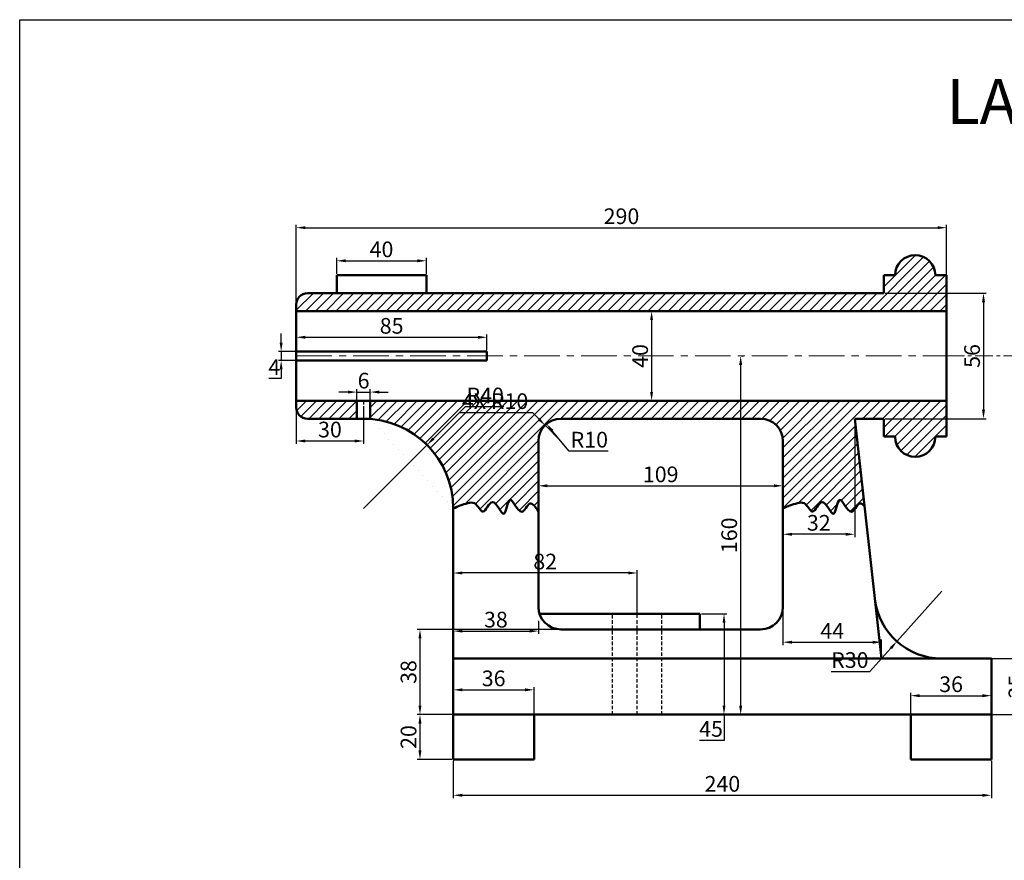
# Model space of a CAD drawing. Units: millimetres. Extents: x -66 to 1195, y -396 to 398.
# Tile 2 of 8: x -66 to 373, y 23 to 398. Entities that reach past the tile are written whole.
import ezdxf

# ---------------------------------------------------------------- set-up
doc = ezdxf.new("R2010")
doc.units = ezdxf.units.MM
doc.header["$LTSCALE"] = 0.5
doc.linetypes.add('CENTER', pattern=[50.8, 31.75, -6.35, 6.35, -6.35])
doc.linetypes.add('HIDDEN', pattern=[9.525, 6.35, -3.175])
for name, color, linetype, lineweight in [('M-CNTR', 1, 'CENTER', 18), ('M-DIMS', 2, 'Continuous', 25), ('M-HATC', 8, 'Continuous', 18), ('M-HIDN', 3, 'HIDDEN', 25), ('M-OUTL', 7, 'Continuous', 50), ('M-TEXT', 7, 'Continuous', 25), ('M-TTLB', 7, 'Continuous', 25)]:
    doc.layers.add(name, color=color, linetype=linetype, lineweight=lineweight)
doc.styles.get("Standard").update_dxf_attribs({"font": 'arial.ttf'})
doc.dimstyles.new('ISO-25', dxfattribs={"dimtxt": 7, "dimasz": 4, "dimexe": 1.25, "dimexo": 0.625, "dimtad": 1, "dimtoh": 1, "dimtxsty": 'Standard', "dimcen": 2.5, "dimadec": 0, "dimazin": 0, "dimtfac": 1, "dimtmove": 0, "dimatfit": 3, "dimfxl": 1, "dimarcsym": 0})

# ---------------------------------------------------------------- blocks, each defined once
blk = doc.blocks.new('*D1')
at = {"layer": 'Defpoints', "color": 0, "ltscale": 0.5, "transparency": 16777216}
for p in [(114.94, 290.08), (74.94, 283.61), (114.94, 283.61)]:
    blk.add_point(p, dxfattribs=at)
at = {"layer": 'M-DIMS', "color": 0, "lineweight": -2, "ltscale": 0.5, "transparency": 16777216}
for p, q in [((74.94, 284.24), (74.94, 291.33)), ((78.94, 290.08), (110.94, 290.08)), ((114.94, 284.24), (114.94, 291.33))]:
    blk.add_line(p, q, dxfattribs=at)
at = {"layer": 'M-DIMS', "color": 0, "ltscale": 0.5, "transparency": 16777216}
for points in [[(78.94, 290.75), (78.94, 289.41), (74.94, 290.08)], [(110.94, 290.75), (110.94, 289.41), (114.94, 290.08)]]:
    blk.add_solid(points, dxfattribs=at)
at = {"layer": 'M-DIMS', "color": 0, "ltscale": 0.5, "transparency": 16777216, "insert": (94.94, 294.28), "char_height": 7, "attachment_point": 5}
blk.add_mtext('40', dxfattribs=at)
blk = doc.blocks.new('*D2')
at = {"layer": 'Defpoints', "color": 0, "ltscale": 0.5, "transparency": 16777216}
for p in [(346.94, 304.84), (56.94, 249.61), (346.94, 247.61)]:
    blk.add_point(p, dxfattribs=at)
at = {"layer": 'M-DIMS', "color": 0, "lineweight": -2, "ltscale": 0.5, "transparency": 16777216}
for p, q in [((56.94, 250.24), (56.94, 306.09)), ((60.94, 304.84), (342.94, 304.84)), ((346.94, 248.24), (346.94, 306.09))]:
    blk.add_line(p, q, dxfattribs=at)
at = {"layer": 'M-DIMS', "color": 0, "ltscale": 0.5, "transparency": 16777216}
for points in [[(60.94, 305.51), (60.94, 304.18), (56.94, 304.84)], [(342.94, 305.51), (342.94, 304.18), (346.94, 304.84)]]:
    blk.add_solid(points, dxfattribs=at)
at = {"layer": 'M-DIMS', "color": 0, "ltscale": 0.5, "transparency": 16777216, "insert": (201.94, 309.04), "char_height": 7, "attachment_point": 5}
blk.add_mtext('290', dxfattribs=at)
blk = doc.blocks.new('*D3')
at = {"layer": 'Defpoints', "color": 0, "ltscale": 0.5, "transparency": 16777216}
for p in [(141.94, 255.95), (56.94, 249.61), (141.94, 249.61)]:
    blk.add_point(p, dxfattribs=at)
at = {"layer": 'M-DIMS', "color": 0, "lineweight": -2, "ltscale": 0.5, "transparency": 16777216}
for p, q in [((56.94, 250.24), (56.94, 257.2)), ((60.94, 255.95), (137.94, 255.95)), ((141.94, 250.24), (141.94, 257.2))]:
    blk.add_line(p, q, dxfattribs=at)
at = {"layer": 'M-DIMS', "color": 0, "ltscale": 0.5, "transparency": 16777216}
for points in [[(60.94, 256.61), (60.94, 255.28), (56.94, 255.95)], [(137.94, 256.61), (137.94, 255.28), (141.94, 255.95)]]:
    blk.add_solid(points, dxfattribs=at)
at = {"layer": 'M-DIMS', "color": 0, "ltscale": 0.5, "transparency": 16777216, "insert": (99.44, 260.15), "char_height": 7, "attachment_point": 5}
blk.add_mtext('85', dxfattribs=at)
blk = doc.blocks.new('*D4')
at = {"layer": 'Defpoints', "color": 0, "ltscale": 0.5, "transparency": 16777216}
for p in [(56.94, 249.61), (50.18, 245.61), (56.94, 245.61)]:
    blk.add_point(p, dxfattribs=at)
at = {"layer": 'M-DIMS', "color": 0, "lineweight": -2, "ltscale": 0.5, "transparency": 16777216}
for p, q in [((50.18, 253.61), (50.18, 257.61)), ((56.31, 249.61), (48.93, 249.61)), ((50.18, 249.61), (50.18, 245.61)), ((56.31, 245.61), (48.93, 245.61)), ((50.18, 241.61), (50.18, 237.61)), ((50.18, 237.61), (44.71, 237.61))]:
    blk.add_line(p, q, dxfattribs=at)
at = {"layer": 'M-DIMS', "color": 0, "ltscale": 0.5, "transparency": 16777216}
for points in [[(49.51, 253.61), (50.84, 253.61), (50.18, 249.61)], [(49.51, 241.61), (50.84, 241.61), (50.18, 245.61)]]:
    blk.add_solid(points, dxfattribs=at)
at = {"layer": 'M-DIMS', "color": 0, "ltscale": 0.5, "transparency": 16777216, "insert": (47.13, 241.74), "char_height": 7, "attachment_point": 5}
blk.add_mtext('4', dxfattribs=at)
blk = doc.blocks.new('*D5')
at = {"layer": 'Defpoints', "color": 0, "ltscale": 0.5, "transparency": 16777216}
for p in [(219.72, 267.61), (215.38, 227.61), (219.72, 227.61)]:
    blk.add_point(p, dxfattribs=at)
at = {"layer": 'M-DIMS', "color": 0, "lineweight": -2, "ltscale": 0.5, "transparency": 16777216}
for p, q in [((219.09, 267.61), (214.13, 267.61)), ((215.38, 263.61), (215.38, 231.61)), ((219.09, 227.61), (214.13, 227.61))]:
    blk.add_line(p, q, dxfattribs=at)
at = {"layer": 'M-DIMS', "color": 0, "ltscale": 0.5, "transparency": 16777216}
for points in [[(214.71, 263.61), (216.04, 263.61), (215.38, 267.61)], [(214.71, 231.61), (216.04, 231.61), (215.38, 227.61)]]:
    blk.add_solid(points, dxfattribs=at)
at = {"layer": 'M-DIMS', "color": 0, "ltscale": 0.5, "transparency": 16777216, "insert": (211.18, 247.61), "char_height": 7, "attachment_point": 5, "rotation": 90}
blk.add_mtext('40', dxfattribs=at)
blk = doc.blocks.new('*D6')
at = {"layer": 'Defpoints', "color": 0, "ltscale": 0.5, "transparency": 16777216}
for p in [(56.94, 224.61), (86.94, 224.61), (86.94, 209.68)]:
    blk.add_point(p, dxfattribs=at)
at = {"layer": 'M-DIMS', "color": 0, "lineweight": -2, "ltscale": 0.5, "transparency": 16777216}
for p, q in [((56.94, 223.99), (56.94, 208.43)), ((86.94, 223.99), (86.94, 208.43)), ((60.94, 209.68), (82.94, 209.68))]:
    blk.add_line(p, q, dxfattribs=at)
at = {"layer": 'M-DIMS', "color": 0, "ltscale": 0.5, "transparency": 16777216}
for points in [[(60.94, 210.35), (60.94, 209.01), (56.94, 209.68)], [(82.94, 210.35), (82.94, 209.01), (86.94, 209.68)]]:
    blk.add_solid(points, dxfattribs=at)
at = {"layer": 'M-DIMS', "color": 0, "ltscale": 0.5, "transparency": 16777216, "insert": (71.94, 213.88), "char_height": 7, "attachment_point": 5}
blk.add_mtext('30', dxfattribs=at)
blk = doc.blocks.new('*D7')
at = {"layer": 'Defpoints', "color": 0, "ltscale": 0.5, "transparency": 16777216}
for p in [(89.94, 231.5), (83.94, 227.61), (89.94, 227.61)]:
    blk.add_point(p, dxfattribs=at)
at = {"layer": 'M-DIMS', "color": 0, "lineweight": -2, "ltscale": 0.5, "transparency": 16777216}
for p, q in [((83.94, 228.24), (83.94, 232.75)), ((89.94, 228.24), (89.94, 232.75)), ((79.94, 231.5), (75.94, 231.5)), ((83.94, 231.5), (89.94, 231.5)), ((93.94, 231.5), (97.94, 231.5))]:
    blk.add_line(p, q, dxfattribs=at)
at = {"layer": 'M-DIMS', "color": 0, "ltscale": 0.5, "transparency": 16777216}
for points in [[(79.94, 232.17), (79.94, 230.84), (83.94, 231.5)], [(93.94, 232.17), (93.94, 230.84), (89.94, 231.5)]]:
    blk.add_solid(points, dxfattribs=at)
at = {"layer": 'M-DIMS', "color": 0, "ltscale": 0.5, "transparency": 16777216, "insert": (86.94, 235.7), "char_height": 7, "attachment_point": 5}
blk.add_mtext('6', dxfattribs=at)
blk = doc.blocks.new('*D8')
at = {"layer": 'Defpoints', "color": 0, "ltscale": 0.5, "transparency": 16777216}
for p in [(305.94, 219.61), (273.94, 199.66), (273.94, 168.06)]:
    blk.add_point(p, dxfattribs=at)
at = {"layer": 'M-DIMS', "color": 0, "lineweight": -2, "ltscale": 0.5, "transparency": 16777216}
for p, q in [((305.94, 218.99), (305.94, 166.81)), ((273.94, 199.04), (273.94, 166.81)), ((301.94, 168.06), (277.94, 168.06))]:
    blk.add_line(p, q, dxfattribs=at)
at = {"layer": 'M-DIMS', "color": 0, "ltscale": 0.5, "transparency": 16777216}
for points in [[(277.94, 168.73), (277.94, 167.39), (273.94, 168.06)], [(301.94, 168.73), (301.94, 167.39), (305.94, 168.06)]]:
    blk.add_solid(points, dxfattribs=at)
at = {"layer": 'M-DIMS', "color": 0, "ltscale": 0.5, "transparency": 16777216, "insert": (289.94, 172.26), "char_height": 7, "attachment_point": 5}
blk.add_mtext('32', dxfattribs=at)
blk = doc.blocks.new('*D9')
at = {"layer": 'Defpoints', "color": 0, "ltscale": 0.5, "transparency": 16777216}
for p in [(273.94, 142.91), (317.94, 119.9), (317.94, 112.61)]:
    blk.add_point(p, dxfattribs=at)
at = {"layer": 'M-DIMS', "color": 0, "lineweight": -2, "ltscale": 0.5, "transparency": 16777216}
for p, q in [((273.94, 142.29), (273.94, 118.65)), ((277.94, 119.9), (313.94, 119.9)), ((317.94, 113.24), (317.94, 121.15))]:
    blk.add_line(p, q, dxfattribs=at)
at = {"layer": 'M-DIMS', "color": 0, "ltscale": 0.5, "transparency": 16777216}
for points in [[(277.94, 120.57), (277.94, 119.24), (273.94, 119.9)], [(313.94, 120.57), (313.94, 119.24), (317.94, 119.9)]]:
    blk.add_solid(points, dxfattribs=at)
at = {"layer": 'M-DIMS', "color": 0, "ltscale": 0.5, "transparency": 16777216, "insert": (295.94, 124.03), "char_height": 7, "attachment_point": 5}
blk.add_mtext('44', dxfattribs=at)
blk = doc.blocks.new('*D10')
at = {"layer": 'Defpoints', "color": 0, "ltscale": 0.5, "transparency": 16777216}
for p in [(126.94, 150.79), (126.94, 130.11), (208.94, 130.11)]:
    blk.add_point(p, dxfattribs=at)
at = {"layer": 'M-DIMS', "color": 0, "lineweight": -2, "ltscale": 0.5, "transparency": 16777216}
for p, q in [((126.94, 130.74), (126.94, 152.04)), ((204.94, 150.79), (130.94, 150.79)), ((208.94, 130.74), (208.94, 152.04))]:
    blk.add_line(p, q, dxfattribs=at)
at = {"layer": 'M-DIMS', "color": 0, "ltscale": 0.5, "transparency": 16777216}
for points in [[(130.94, 151.46), (130.94, 150.12), (126.94, 150.79)], [(204.94, 151.46), (204.94, 150.12), (208.94, 150.79)]]:
    blk.add_solid(points, dxfattribs=at)
at = {"layer": 'M-DIMS', "color": 0, "ltscale": 0.5, "transparency": 16777216, "insert": (167.94, 154.99), "char_height": 7, "attachment_point": 5}
blk.add_mtext('82', dxfattribs=at)
blk = doc.blocks.new('*D11')
at = {"layer": 'Defpoints', "color": 0, "ltscale": 0.5, "transparency": 16777216}
for p in [(126.94, 130.11), (164.94, 130.11), (164.94, 124.87)]:
    blk.add_point(p, dxfattribs=at)
at = {"layer": 'M-DIMS', "color": 0, "lineweight": -2, "ltscale": 0.5, "transparency": 16777216}
for p, q in [((126.94, 129.49), (126.94, 123.62)), ((164.94, 129.49), (164.94, 123.62)), ((130.94, 124.87), (160.94, 124.87))]:
    blk.add_line(p, q, dxfattribs=at)
at = {"layer": 'M-DIMS', "color": 0, "ltscale": 0.5, "transparency": 16777216}
for points in [[(130.94, 125.53), (130.94, 124.2), (126.94, 124.87)], [(160.94, 125.53), (160.94, 124.2), (164.94, 124.87)]]:
    blk.add_solid(points, dxfattribs=at)
at = {"layer": 'M-DIMS', "color": 0, "ltscale": 0.5, "transparency": 16777216, "insert": (145.94, 129.07), "char_height": 7, "attachment_point": 5}
blk.add_mtext('38', dxfattribs=at)
blk = doc.blocks.new('*D12')
at = {"layer": 'Defpoints', "color": 0, "ltscale": 0.5, "transparency": 16777216}
for p in [(254.81, 247.61), (254.81, 87.61), (255.09, 87.61)]:
    blk.add_point(p, dxfattribs=at)
at = {"layer": 'M-DIMS', "color": 0, "lineweight": -2, "ltscale": 0.5, "transparency": 16777216}
for p, q in [((255.43, 247.61), (256.34, 247.61)), ((255.09, 243.61), (255.09, 91.61)), ((255.43, 87.61), (256.34, 87.61))]:
    blk.add_line(p, q, dxfattribs=at)
at = {"layer": 'M-DIMS', "color": 0, "ltscale": 0.5, "transparency": 16777216}
for points in [[(254.42, 243.61), (255.76, 243.61), (255.09, 247.61)], [(254.42, 91.61), (255.76, 91.61), (255.09, 87.61)]]:
    blk.add_solid(points, dxfattribs=at)
at = {"layer": 'M-DIMS', "color": 0, "ltscale": 0.5, "transparency": 16777216, "insert": (250.89, 167.61), "char_height": 7, "attachment_point": 5, "rotation": 90}
blk.add_mtext('160', dxfattribs=at)
blk = doc.blocks.new('*D13')
at = {"layer": 'Defpoints', "color": 0, "ltscale": 0.5, "transparency": 16777216}
for p in [(273.94, 189.69), (164.94, 188.31), (273.94, 188.31)]:
    blk.add_point(p, dxfattribs=at)
at = {"layer": 'M-DIMS', "color": 0, "lineweight": -2, "ltscale": 0.5, "transparency": 16777216}
for p, q in [((164.94, 188.93), (164.94, 190.94)), ((168.94, 189.69), (269.94, 189.69)), ((273.94, 188.93), (273.94, 190.94))]:
    blk.add_line(p, q, dxfattribs=at)
at = {"layer": 'M-DIMS', "color": 0, "ltscale": 0.5, "transparency": 16777216}
for points in [[(168.94, 190.35), (168.94, 189.02), (164.94, 189.69)], [(269.94, 190.35), (269.94, 189.02), (273.94, 189.69)]]:
    blk.add_solid(points, dxfattribs=at)
at = {"layer": 'M-DIMS', "color": 0, "ltscale": 0.5, "transparency": 16777216, "insert": (219.44, 193.89), "char_height": 7, "attachment_point": 5}
blk.add_mtext('109', dxfattribs=at)
blk = doc.blocks.new('*D14')
at = {"layer": 'Defpoints', "color": 0, "ltscale": 0.5, "transparency": 16777216}
for p in [(168.54, 217.3), (174.94, 209.61)]:
    blk.add_point(p, dxfattribs=at)
at = {"layer": 'M-DIMS', "color": 0, "lineweight": -2, "ltscale": 0.5, "transparency": 16777216}
for p, q in [((178.64, 205.16), (171.1, 214.22)), ((195.96, 205.16), (178.64, 205.16))]:
    blk.add_line(p, q, dxfattribs=at)
at = {"layer": 'M-DIMS', "color": 0, "ltscale": 0.5, "transparency": 16777216}
blk.add_solid([(171.61, 214.65), (170.59, 213.8), (168.54, 217.3)], dxfattribs=at)
at = {"layer": 'M-DIMS', "color": 0, "ltscale": 0.5, "transparency": 16777216, "insert": (187.61, 209.36), "char_height": 7, "attachment_point": 5}
blk.add_mtext('R10', dxfattribs=at)
blk = doc.blocks.new('*D15')
at = {"layer": 'Defpoints', "color": 0, "ltscale": 0.5, "transparency": 16777216}
for p in [(181.38, 125.61), (112.09, 87.61), (181.38, 87.61)]:
    blk.add_point(p, dxfattribs=at)
at = {"layer": 'M-DIMS', "color": 0, "lineweight": -2, "ltscale": 0.5, "transparency": 16777216}
for p, q in [((180.75, 125.61), (110.84, 125.61)), ((112.09, 121.61), (112.09, 91.61)), ((180.75, 87.61), (110.84, 87.61))]:
    blk.add_line(p, q, dxfattribs=at)
at = {"layer": 'M-DIMS', "color": 0, "ltscale": 0.5, "transparency": 16777216}
for points in [[(111.42, 121.61), (112.75, 121.61), (112.09, 125.61)], [(111.42, 91.61), (112.75, 91.61), (112.09, 87.61)]]:
    blk.add_solid(points, dxfattribs=at)
at = {"layer": 'M-DIMS', "color": 0, "ltscale": 0.5, "transparency": 16777216, "insert": (107.89, 106.61), "char_height": 7, "attachment_point": 5, "rotation": 90}
blk.add_mtext('38', dxfattribs=at)
blk = doc.blocks.new('*D16')
at = {"layer": 'Defpoints', "color": 0, "ltscale": 0.5, "transparency": 16777216}
for p in [(126.94, 87.61), (112.09, 67.61), (126.94, 67.61)]:
    blk.add_point(p, dxfattribs=at)
at = {"layer": 'M-DIMS', "color": 0, "lineweight": -2, "ltscale": 0.5, "transparency": 16777216}
for p, q in [((126.31, 87.61), (110.84, 87.61)), ((112.09, 83.61), (112.09, 71.61)), ((126.31, 67.61), (110.84, 67.61))]:
    blk.add_line(p, q, dxfattribs=at)
at = {"layer": 'M-DIMS', "color": 0, "ltscale": 0.5, "transparency": 16777216}
for points in [[(111.42, 83.61), (112.75, 83.61), (112.09, 87.61)], [(111.42, 71.61), (112.75, 71.61), (112.09, 67.61)]]:
    blk.add_solid(points, dxfattribs=at)
at = {"layer": 'M-DIMS', "color": 0, "ltscale": 0.5, "transparency": 16777216, "insert": (107.89, 77.61), "char_height": 7, "attachment_point": 5, "rotation": 90}
blk.add_mtext('20', dxfattribs=at)
blk = doc.blocks.new('*D17')
at = {"layer": 'Defpoints', "color": 0, "ltscale": 0.5, "transparency": 16777216}
for p in [(236.94, 132.61), (236.94, 87.61), (247.68, 87.61)]:
    blk.add_point(p, dxfattribs=at)
at = {"layer": 'M-DIMS', "color": 0, "lineweight": -2, "ltscale": 0.5, "transparency": 16777216}
for p, q in [((237.56, 132.61), (248.93, 132.61)), ((247.68, 128.61), (247.68, 91.61)), ((237.56, 87.61), (248.93, 87.61)), ((247.68, 87.61), (247.68, 76.13)), ((247.68, 76.13), (236.69, 76.13))]:
    blk.add_line(p, q, dxfattribs=at)
at = {"layer": 'M-DIMS', "color": 0, "ltscale": 0.5, "transparency": 16777216}
for points in [[(247.01, 128.61), (248.34, 128.61), (247.68, 132.61)], [(247.01, 91.61), (248.34, 91.61), (247.68, 87.61)]]:
    blk.add_solid(points, dxfattribs=at)
at = {"layer": 'M-DIMS', "color": 0, "ltscale": 0.5, "transparency": 16777216, "insert": (241.87, 80.32), "char_height": 7, "attachment_point": 5}
blk.add_mtext('45', dxfattribs=at)
blk = doc.blocks.new('*D18')
at = {"layer": 'Defpoints', "color": 0, "ltscale": 0.5, "transparency": 16777216}
for p in [(126.94, 67.61), (366.94, 67.61), (366.94, 51.62)]:
    blk.add_point(p, dxfattribs=at)
at = {"layer": 'M-DIMS', "color": 0, "lineweight": -2, "ltscale": 0.5, "transparency": 16777216}
for p, q in [((126.94, 66.99), (126.94, 50.37)), ((366.94, 66.99), (366.94, 50.37)), ((130.94, 51.62), (362.94, 51.62))]:
    blk.add_line(p, q, dxfattribs=at)
at = {"layer": 'M-DIMS', "color": 0, "ltscale": 0.5, "transparency": 16777216}
for points in [[(130.94, 52.28), (130.94, 50.95), (126.94, 51.62)], [(362.94, 52.28), (362.94, 50.95), (366.94, 51.62)]]:
    blk.add_solid(points, dxfattribs=at)
at = {"layer": 'M-DIMS', "color": 0, "ltscale": 0.5, "transparency": 16777216, "insert": (246.94, 55.82), "char_height": 7, "attachment_point": 5}
blk.add_mtext('240', dxfattribs=at)
blk = doc.blocks.new('*D19')
at = {"layer": 'Defpoints', "color": 0, "ltscale": 0.5, "transparency": 16777216}
for p in [(162.94, 98.67), (126.94, 87.61), (162.94, 87.61)]:
    blk.add_point(p, dxfattribs=at)
at = {"layer": 'M-DIMS', "color": 0, "lineweight": -2, "ltscale": 0.5, "transparency": 16777216}
for p, q in [((126.94, 88.24), (126.94, 99.92)), ((130.94, 98.67), (158.94, 98.67)), ((162.94, 88.24), (162.94, 99.92))]:
    blk.add_line(p, q, dxfattribs=at)
at = {"layer": 'M-DIMS', "color": 0, "ltscale": 0.5, "transparency": 16777216}
for points in [[(130.94, 99.33), (130.94, 98), (126.94, 98.67)], [(158.94, 99.33), (158.94, 98), (162.94, 98.67)]]:
    blk.add_solid(points, dxfattribs=at)
at = {"layer": 'M-DIMS', "color": 0, "ltscale": 0.5, "transparency": 16777216, "insert": (144.94, 102.87), "char_height": 7, "attachment_point": 5}
blk.add_mtext('36', dxfattribs=at)
blk = doc.blocks.new('*D20')
at = {"layer": 'Defpoints', "color": 0, "ltscale": 0.5, "transparency": 16777216}
for p in [(366.94, 96.06), (330.94, 87.61), (366.94, 87.61)]:
    blk.add_point(p, dxfattribs=at)
at = {"layer": 'M-DIMS', "color": 0, "lineweight": -2, "ltscale": 0.5, "transparency": 16777216}
for p, q in [((330.94, 88.24), (330.94, 97.31)), ((366.94, 88.24), (366.94, 97.31)), ((334.94, 96.06), (362.94, 96.06))]:
    blk.add_line(p, q, dxfattribs=at)
at = {"layer": 'M-DIMS', "color": 0, "ltscale": 0.5, "transparency": 16777216}
for points in [[(334.94, 96.73), (334.94, 95.39), (330.94, 96.06)], [(362.94, 96.73), (362.94, 95.39), (366.94, 96.06)]]:
    blk.add_solid(points, dxfattribs=at)
at = {"layer": 'M-DIMS', "color": 0, "ltscale": 0.5, "transparency": 16777216, "insert": (348.94, 100.26), "char_height": 7, "attachment_point": 5}
blk.add_mtext('36', dxfattribs=at)
blk = doc.blocks.new('*D21')
at = {"layer": 'Defpoints', "color": 0, "ltscale": 0.5, "transparency": 16777216}
for p in [(318.94, 275.61), (318.94, 219.61), (363.39, 219.61)]:
    blk.add_point(p, dxfattribs=at)
at = {"layer": 'M-DIMS', "color": 0, "lineweight": -2, "ltscale": 0.5, "transparency": 16777216}
for p, q in [((319.56, 275.61), (364.64, 275.61)), ((363.39, 271.61), (363.39, 223.61)), ((319.56, 219.61), (364.64, 219.61))]:
    blk.add_line(p, q, dxfattribs=at)
at = {"layer": 'M-DIMS', "color": 0, "ltscale": 0.5, "transparency": 16777216}
for points in [[(362.73, 271.61), (364.06, 271.61), (363.39, 275.61)], [(362.73, 223.61), (364.06, 223.61), (363.39, 219.61)]]:
    blk.add_solid(points, dxfattribs=at)
at = {"layer": 'M-DIMS', "color": 0, "ltscale": 0.5, "transparency": 16777216, "insert": (359.2, 247.61), "char_height": 7, "attachment_point": 5, "rotation": 90}
blk.add_mtext('56', dxfattribs=at)
blk = doc.blocks.new('*D30')
at = {"layer": 'Defpoints', "color": 0, "ltscale": 0.5, "transparency": 16777216}
for p in [(185.07, 112.61), (185.07, 87.61), (383.19, 87.61)]:
    blk.add_point(p, dxfattribs=at)
at = {"layer": 'M-DIMS', "color": 0, "lineweight": -2, "ltscale": 0.5, "transparency": 16777216}
for p, q in [((185.69, 112.61), (384.44, 112.61)), ((383.19, 108.61), (383.19, 91.61)), ((185.69, 87.61), (384.44, 87.61))]:
    blk.add_line(p, q, dxfattribs=at)
at = {"layer": 'M-DIMS', "color": 0, "ltscale": 0.5, "transparency": 16777216}
for points in [[(382.52, 108.61), (383.85, 108.61), (383.19, 112.61)], [(382.52, 91.61), (383.85, 91.61), (383.19, 87.61)]]:
    blk.add_solid(points, dxfattribs=at)
at = {"layer": 'M-DIMS', "color": 0, "ltscale": 0.5, "transparency": 16777216, "insert": (378.99, 100.11), "char_height": 7, "attachment_point": 5, "rotation": 90}
blk.add_mtext('25', dxfattribs=at)
blk = doc.blocks.new('*D115')
at = {"layer": 'Defpoints', "color": 0, "ltscale": 0.5, "transparency": 16777216}
for p in [(115.22, 207.9), (86.94, 179.61)]:
    blk.add_point(p, dxfattribs=at)
at = {"layer": 'M-DIMS', "color": 0, "lineweight": -2, "ltscale": 0.5, "transparency": 16777216}
for p, q in [((132.19, 224.87), (118.05, 210.73)), ((149.51, 224.87), (132.19, 224.87)), ((86.94, 179.61), (115.22, 207.9))]:
    blk.add_line(p, q, dxfattribs=at)
at = {"layer": 'M-DIMS', "color": 0, "ltscale": 0.5, "transparency": 16777216}
blk.add_solid([(117.57, 211.2), (118.52, 210.26), (115.22, 207.9)], dxfattribs=at)
at = {"layer": 'M-DIMS', "color": 0, "ltscale": 0.5, "transparency": 16777216, "insert": (141.16, 229.07), "char_height": 7, "attachment_point": 5}
blk.add_mtext('R40', dxfattribs=at)
blk = doc.blocks.new('*D116')
at = {"layer": 'Defpoints', "color": 0, "ltscale": 0.5, "transparency": 16777216}
for p in [(344.76, 142.61), (324.76, 120.25)]:
    blk.add_point(p, dxfattribs=at)
at = {"layer": 'M-DIMS', "color": 0, "lineweight": -2, "ltscale": 0.5, "transparency": 16777216}
for p, q in [((344.76, 142.61), (324.76, 120.25)), ((312.76, 106.83), (322.09, 117.27)), ((295.43, 106.83), (312.76, 106.83))]:
    blk.add_line(p, q, dxfattribs=at)
at = {"layer": 'M-DIMS', "color": 0, "ltscale": 0.5, "transparency": 16777216}
blk.add_solid([(321.6, 117.71), (322.59, 116.82), (324.76, 120.25)], dxfattribs=at)
at = {"layer": 'M-DIMS', "color": 0, "ltscale": 0.5, "transparency": 16777216, "insert": (303.78, 111.04), "char_height": 7, "attachment_point": 5}
blk.add_mtext('R30', dxfattribs=at)
blk = doc.blocks.new('*D117')
at = {"layer": 'Defpoints', "color": 0, "ltscale": 0.5, "transparency": 16777216}
for p in [(167.87, 216.68), (174.94, 209.61)]:
    blk.add_point(p, dxfattribs=at)
at = {"layer": 'M-DIMS', "color": 0, "lineweight": -2, "ltscale": 0.5, "transparency": 16777216}
for p, q in [((129.56, 222.34), (162.21, 222.34)), ((162.21, 222.34), (165.04, 219.51)), ((174.94, 209.61), (167.87, 216.68))]:
    blk.add_line(p, q, dxfattribs=at)
at = {"layer": 'M-DIMS', "color": 0, "ltscale": 0.5, "transparency": 16777216}
blk.add_solid([(165.51, 219.98), (164.57, 219.04), (167.87, 216.68)], dxfattribs=at)
at = {"layer": 'M-DIMS', "color": 0, "ltscale": 0.5, "transparency": 16777216, "insert": (145.57, 226.54), "char_height": 7, "attachment_point": 5}
blk.add_mtext('4X R10', dxfattribs=at)

msp = doc.modelspace()

# ---------------------------------------------------------------- hatches: boundary and pattern name
at = {"layer": 'M-HATC', "ltscale": 0.5}
h = msp.add_hatch(dxfattribs=at)
h.set_pattern_fill('ANSI31', color=256)
h.paths.add_polyline_path([(346.9367, 283.6106), (341.9367, 283.6106, 1), (323.9367, 283.6106), (318.9367, 283.6106), (318.9367, 275.6106), (61.9367, 275.6106, 0.41421356), (56.9367, 270.6106), (56.9367, 267.6106), (346.9367, 267.6106)])
edge = h.paths.add_edge_path()
edge.add_arc((174.9367, 209.6106), 10, 90, 180, ccw=False)
edge.add_line((174.9367, 219.6106), (263.9367, 219.6106))
edge.add_arc((263.9367, 209.6106), 10, 0, 90, ccw=False)
edge.add_line((273.9367, 209.6106), (273.9367, 179.6106))
edge.add_spline(control_points=[(273.9367, 179.6106), (276.0021, 180.4667), (278.9643, 181.6945), (284.4139, 182.7709), (287.1838, 174.6918), (291.5759, 187.2), (297.2165, 171.6922), (298.5298, 189.0126), (304.0806, 173.9252), (307.5276, 182.9887), (309.5476, 181.4788), (310.3171, 180.5517)], knot_values=[0, 0, 0, 0, 6.87842387, 9.86491468, 15.17570471, 21.17110582, 28.46043275, 35.12417976, 42.54660911, 47.65719912, 50.72137428, 50.72137428, 50.72137428, 50.72137428], degree=3, periodic=0)
edge.add_line((310.3171, 180.5517), (305.9367, 219.6106))
edge.add_line((305.9367, 219.6106), (318.9367, 219.6106))
edge.add_line((318.9367, 219.6106), (318.9367, 211.6106))
edge.add_line((318.9367, 211.6106), (323.9367, 211.6106))
edge.add_arc((332.9367, 211.6106), 9, 180, 360)
edge.add_line((341.9367, 211.6106), (346.9367, 211.6106))
edge.add_line((346.9367, 211.6106), (346.9367, 227.6106))
edge.add_line((346.9367, 227.6106), (89.9367, 227.6106))
edge.add_line((89.9367, 227.6106), (89.9367, 219.4979))
edge.add_arc((86.9367, 179.6106), 40, 0, 85.698778, ccw=False)
edge.add_spline(control_points=[(126.9367, 179.6106), (129.0021, 180.4667), (131.9643, 181.6945), (137.4139, 182.7709), (140.1838, 174.6918), (144.5759, 187.2), (150.2165, 171.6922), (151.5298, 189.0126), (157.0806, 173.9252), (160.9991, 184.2287), (163.6168, 180.2639), (164.9367, 178.2647)], knot_values=[0, 0, 0, 0, 6.87842387, 9.86491468, 15.17570471, 21.17110582, 28.46043275, 35.12417976, 42.54660911, 47.65719912, 52.85524611, 52.85524611, 52.85524611, 52.85524611], degree=3, periodic=0)
edge.add_line((164.9367, 178.2647), (164.9367, 209.6106))
h.paths.add_polyline_path([(83.9367, 227.6106), (56.9367, 227.6106), (56.9367, 224.6106, 0.41421356), (61.9367, 219.6106), (83.9367, 219.6106)])

# ---------------------------------------------------------------- linework, layer by layer
at = {"layer": 'M-CNTR'}
msp.add_line((56.9367, 247.6106), (346.9367, 247.6106), dxfattribs=at)
at = {"layer": 'M-CNTR', "ltscale": 0.5}
msp.add_line((346.9367, 247.6106), (539.9794, 247.6106), dxfattribs=at)
at = {"layer": 'M-HIDN', "ltscale": 0.5}
for p, q in [((86.9367, 227.6106), (86.9367, 219.6106)), ((197.9367, 87.6106), (197.9367, 132.6106)), ((219.9367, 87.6106), (219.9367, 132.6106)), ((208.9367, 87.6106), (208.9367, 130.1106))]:
    msp.add_line(p, q, dxfattribs=at)
at = {"layer": 'M-OUTL', "ltscale": 0.5}
for p, q in [((114.9367, 283.6106), (74.9367, 283.6106)), ((74.9367, 275.6106), (74.9367, 283.6106)), ((114.9367, 275.6106), (114.9367, 283.6106)), ((323.9367, 283.6106), (318.9367, 283.6106)), ((318.9367, 283.6106), (318.9367, 275.6106)), ((346.9367, 283.6106), (341.9367, 283.6106)), ((346.9367, 211.6106), (346.9367, 283.6106)), ((56.9367, 249.6106), (141.9367, 249.6106)), ((56.9367, 245.6106), (56.9367, 249.6106)), ((141.9367, 249.6106), (141.9367, 245.6106)), ((141.9367, 245.6106), (56.9367, 245.6106)), ((83.9367, 227.6106), (83.9367, 219.6106)), ((89.9367, 227.6106), (89.9367, 219.6106)), ((305.9367, 219.6106), (318.9367, 219.6106)), ((317.9367, 112.6106), (305.9367, 219.6106)), ((318.9367, 219.6106), (318.9367, 211.6106)), ((318.9367, 211.6106), (323.9367, 211.6106)), ((341.9367, 211.6106), (346.9367, 211.6106)), ((164.9367, 135.6106), (164.9367, 209.6106)), ((273.9367, 135.6106), (273.9367, 209.6106)), ((126.9367, 112.6106), (126.9367, 179.6106)), ((165.3973, 132.6106), (236.9367, 132.6106)), ((236.9367, 125.6106), (236.9367, 132.6106)), ((174.9367, 125.6106), (263.9367, 125.6106))]:
    msp.add_line(p, q, dxfattribs=at)
at = {"layer": 'M-OUTL'}
for p, q in [((61.9367, 275.6106), (318.9367, 275.6106)), ((346.9367, 275.6106), (346.9367, 219.6106)), ((56.9367, 224.6106), (56.9367, 270.6106)), ((56.9367, 267.6106), (346.9367, 267.6106)), ((56.9367, 227.6106), (346.9367, 227.6106)), ((61.9367, 219.6106), (89.9367, 219.6106)), ((174.9367, 219.6106), (263.9367, 219.6106)), ((366.9367, 112.6106), (126.9367, 112.6106)), ((126.9367, 112.6106), (126.9367, 87.6106)), ((366.9367, 87.6106), (366.9367, 112.6106)), ((126.9367, 87.6106), (366.9367, 87.6106)), ((126.9367, 87.6106), (126.9367, 67.6106)), ((162.9367, 67.6106), (162.9367, 87.6106)), ((330.9367, 67.6106), (330.9367, 87.6106)), ((366.9367, 87.6106), (366.9367, 67.6106)), ((126.9367, 67.6106), (162.9367, 67.6106)), ((366.9367, 67.6106), (330.9367, 67.6106))]:
    msp.add_line(p, q, dxfattribs=at)
at = {"layer": 'M-OUTL', "ltscale": 0.5}
for centre, radius, start, end in [((332.9367, 283.6106), 9, 0, 180), ((86.9367, 179.6106), 40, 0, 90), ((174.9367, 209.6106), 10, 90, 180), ((263.9367, 209.6106), 10, 0, 90), ((332.9367, 211.6106), 9, 180, 0), ((344.7603, 142.6106), 30, 186.398957, 270), ((174.9367, 135.6106), 10, 180, 270), ((263.9367, 135.6106), 10, 270, 0)]:
    msp.add_arc(centre, radius, start, end, dxfattribs=at)
at = {"layer": 'M-OUTL'}
for centre, start, end in [((61.9367, 270.6106), 90, 180), ((61.9367, 224.6106), 180, 270)]:
    msp.add_arc(centre, 5, start, end, dxfattribs=at)
at = {"layer": 'M-OUTL', "ltscale": 0.5}
for points, knots in [([(126.9367, 179.6106), (129.0021, 180.4667), (131.9643, 181.6945), (137.4139, 182.7709), (140.1838, 174.6918), (144.5759, 187.2), (150.2165, 171.6922), (151.5298, 189.0126), (157.0806, 173.9252), (160.9991, 184.2287), (163.6168, 180.2639), (164.9367, 178.2647)], [0, 0, 0, 0, 6.87842387, 9.86491468, 15.17570471, 21.17110582, 28.46043275, 35.12417976, 42.54660911, 47.65719912, 52.85524611, 52.85524611, 52.85524611, 52.85524611]), ([(273.9367, 179.6106), (276.0021, 180.4667), (278.9643, 181.6945), (284.4139, 182.7709), (287.1838, 174.6918), (291.5759, 187.2), (297.2165, 171.6922), (298.5298, 189.0126), (304.0806, 173.9252), (307.5276, 182.9887), (309.5476, 181.4788), (310.3171, 180.5517)], [0, 0, 0, 0, 6.87842387, 9.86491468, 15.17570471, 21.17110582, 28.46043275, 35.12417976, 42.54660911, 47.65719912, 50.72137428, 50.72137428, 50.72137428, 50.72137428])]:
    msp.add_open_spline(points, degree=3, knots=knots, dxfattribs=at)
at = {"layer": 'M-TTLB', "ltscale": 0.5}
msp.add_lwpolyline([(-66.4176, 397.641), (1195.0519, 397.641), (1195.0519, -395.6964), (-66.4176, -395.6964)], close=True, dxfattribs=at)

# ---------------------------------------------------------------- texts
at = {"layer": 'M-TEXT', "ltscale": 0.5, "insert": (346.8576, 371.1482), "char_height": 20, "attachment_point": 1}
msp.add_mtext_dynamic_manual_height_columns('LATHE TAIL STOCK COMPONENTS ', width=485.790741, gutter_width=12.5, heights=[0], dxfattribs=at)

# ---------------------------------------------------------------- dimensions: what is measured, and where the dimension line sits
at = {"layer": 'M-DIMS', "ltscale": 0.5}
for base, p1, p2, picture, middle in [((346.9367, 304.843), (56.9367, 249.6106), (346.9367, 247.6106), '*D2', (201.9367, 309.042)), ((114.9367, 290.0799), (74.9367, 283.6106), (114.9367, 283.6106), '*D1', (94.9367, 294.279)), ((141.9367, 255.948), (56.9367, 249.6106), (141.9367, 249.6106), '*D3', (99.4367, 260.147)), ((89.9367, 231.503), (83.9367, 227.6106), (89.9367, 227.6106), '*D7', (86.9367, 235.702)), ((86.9367, 209.6799), (56.9367, 224.6106), (86.9367, 224.6106), '*D6', (71.9367, 213.8813)), ((273.9367, 168.0598), (305.9367, 219.6106), (273.9367, 199.6642), '*D8', (289.9367, 172.2612)), ((273.9367, 189.6871), (164.9367, 188.3081), (273.9367, 188.3081), '*D13', (219.4367, 193.8861)), ((126.9367, 150.7912), (208.9367, 130.1106), (126.9367, 130.1106), '*D10', (167.9367, 154.9902)), ((317.9367, 119.905), (273.9367, 142.9121), (317.9367, 112.6106), '*D9', (295.9367, 124.03)), ((164.9367, 124.8657), (126.9367, 130.1106), (164.9367, 130.1106), '*D11', (145.9367, 129.0671)), ((366.9367, 96.06), (330.9367, 87.6106), (366.9367, 87.6106), '*D20', (348.9367, 100.2614)), ((366.9367, 51.6173), (126.9367, 67.6106), (366.9367, 67.6106), '*D18', (246.9367, 55.8163))]:
    dim = msp.add_linear_dim(base=base, p1=p1, p2=p2, dimstyle='ISO-25', override={"dimclrd": 0, "dimclre": 0, "dimclrt": 0}, dxfattribs=at)
    dim.commit()
    dim.dimension.update_dxf_attribs({"geometry": picture, "text_midpoint": middle})
for base, p1, p2, picture, middle in [((363.3941, 219.6106), (318.9367, 275.6106), (318.9367, 219.6106), '*D21', (359.1951, 247.6106)), ((215.3757, 227.6106), (219.7196, 267.6106), (219.7196, 227.6106), '*D5', (211.1767, 247.6106)), ((50.1751, 245.6106), (56.9367, 249.6106), (56.9367, 245.6106), '*D4', (47.1292, 241.7356)), ((255.0884, 87.6106), (254.8098, 247.6106), (254.8098, 87.6106), '*D12', (250.8894, 167.6106)), ((112.0882, 87.6106), (181.3778, 125.6106), (181.3778, 87.6106), '*D15', (107.8868, 106.6106)), ((383.1852, 87.6106), (185.0679, 112.6106), (185.0679, 87.6106), '*D30', (378.9862, 100.1106)), ((112.0882, 67.6106), (126.9367, 87.6106), (126.9367, 67.6106), '*D16', (107.8892, 77.6106))]:
    dim = msp.add_linear_dim(base=base, p1=p1, p2=p2, angle=90, dimstyle='ISO-25', override={"dimclrd": 0, "dimclre": 0, "dimclrt": 0}, dxfattribs=at)
    dim.commit()
    dim.dimension.update_dxf_attribs({"geometry": picture, "text_midpoint": middle})
for center, mpoint, override, picture, middle in [((86.9367, 179.6106), (115.2179, 207.8979), {"dimdec": 0, "dimlfac": 1, "dimrnd": 0, "dimzin": 0, "dimdsep": 46, "dimlunit": 2}, '*D115', (141.1629, 224.8703)), ((174.9367, 209.6106), (168.5406, 217.2976), {"dimclrd": 0, "dimclre": 0, "dimclrt": 0}, '*D14', (187.612, 205.165)), ((344.7603, 142.6106), (324.7601, 120.2501), {"dimdec": 0, "dimlfac": 1, "dimrnd": 0, "dimzin": 0, "dimdsep": 46, "dimlunit": 2}, '*D116', (303.7837, 106.8338))]:
    dim = msp.add_radius_dim(center=center, mpoint=mpoint, dimstyle='ISO-25', override=override, dxfattribs=at)
    dim.commit()
    dim.dimension.update_dxf_attribs({"geometry": picture, "text_midpoint": middle, "dimtype": 164})
dim = msp.add_radius_dim(center=(174.9367, 209.6106), mpoint=(167.867, 216.683), text='4X <>', dimstyle='ISO-25', override={"dimdec": 0, "dimlfac": 1, "dimrnd": 0, "dimzin": 0, "dimdsep": 46, "dimlunit": 2}, dxfattribs=at)
dim.commit()
dim.dimension.update_dxf_attribs({"geometry": '*D117', "text_midpoint": (145.5736, 226.54)})
dim = msp.add_linear_dim(base=(247.6768, 87.6106), p1=(236.9367, 132.6106), p2=(236.9367, 87.6106), angle=90, dimstyle='ISO-25', override={"dimclrd": 0, "dimclre": 0, "dimclrt": 0}, dxfattribs=at)
dim.commit()
dim.dimension.update_dxf_attribs({"geometry": '*D17', "text_midpoint": (241.871, 76.1334), "dimtype": 160})
dim = msp.add_linear_dim(base=(162.9367, 98.6678), p1=(126.9367, 87.6106), p2=(162.9367, 87.6106), dimstyle='ISO-25', override={"dimclrd": 0, "dimclre": 0, "dimclrt": 0}, dxfattribs=at)
dim.commit()
dim.dimension.update_dxf_attribs({"geometry": '*D19', "text_midpoint": (144.9367, 98.6678), "dimtype": 160})

doc.saveas('drawing.dxf')
